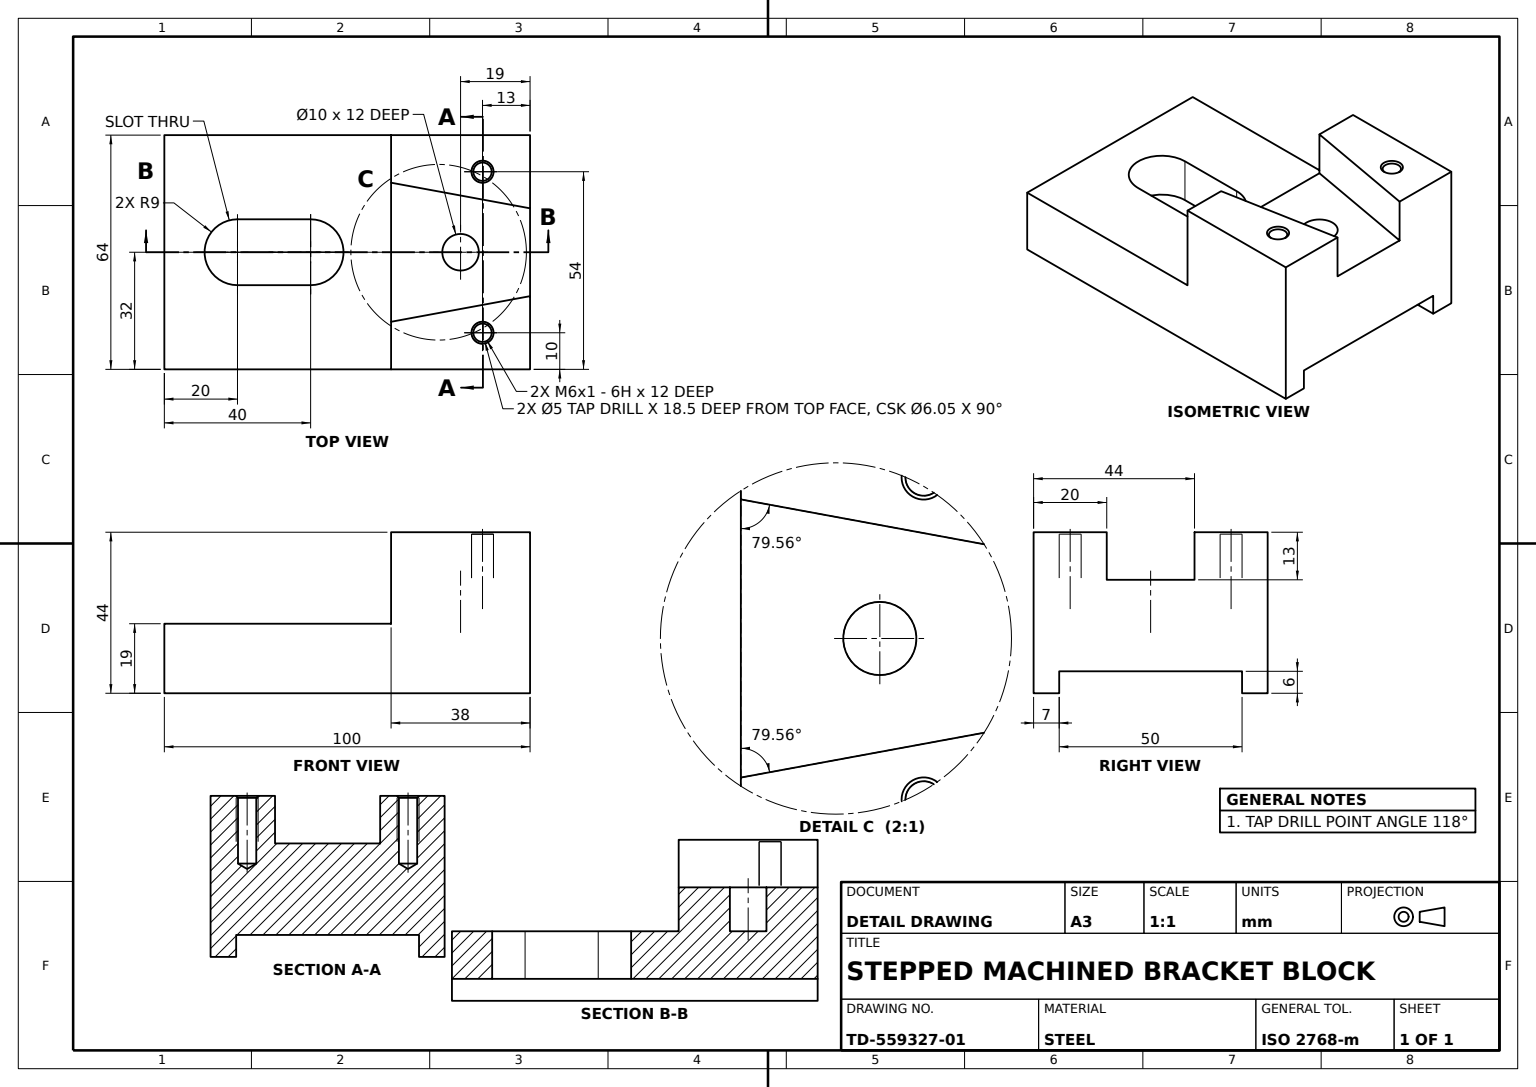
SolidWorks part; units mm, degrees
material "Plain Carbon Steel"
ref_plane "Front Plane" through (0, 0, 0) normal (0, 0, 1) x (1, 0, 0)
ref_plane "Top Plane" through (0, 0, 0) normal (0, 1, 0) x (1, 0, 0)
ref_plane "Right Plane" through (0, 0, 0) normal (1, 0, 0) x (0, 0, -1)
sketch "Base Plate Profile" plane through (0, 0, 0) normal (0, 0, 1) x (1, 0, 0)
  line L0 (25, 0) -> (-25, 0)
  line L1 (-25, 0) -> (-25, -6)
  line L2 (-25, -6) -> (-32, -6)
  line L3 (-32, -6) -> (-32, 13)
  line L4 (-32, 13) -> (32, 13)
  line L5 (32, 13) -> (32, -6)
  line L6 (32, -6) -> (25, -6)
  line L7 (25, -6) -> (25, 0)
  point P4 (0, 0)
  dimension "D1" = 50
  dimension "D2" = 19
  dimension "D3" = 7
  dimension "D4" = 6
  dimension "D5" = 6
  dimension "D6" = 7
  dimension "D7" = 64
extrude "Base Plate" add sketch "Base Plate Profile" against normal blind 100
sketch "V-Block Uprights Profile" plane through (0, 13, 0) normal (0, 1, 0) x (1, 0, 0)
  line L0 (32, 100) -> (32, 62)
  line L1 (32, 100) -> (32, 0) construction
  line L2 (32, 62) -> (19, 62)
  line L3 (19, 62) -> (12, 100)
  line L4 (32, 100) -> (-32, 100) construction
  line L5 (12, 100) -> (32, 100)
  line L6 (0, -24.2) -> (0, 24.2) construction
  line L7 (-12, 100) -> (-32, 100)
  line L8 (-32, 100) -> (-32, 62)
  line L9 (-32, 62) -> (-19, 62)
  line L10 (-19, 62) -> (-12, 100)
  dimension "D1" = 13
  dimension "D2" = 38
  dimension "D3" = 20
extrude "V-Block Uprights" add sketch "V-Block Uprights Profile" along normal blind 25
hole_wizard "M6 Tapped Holes 2x" positions "Sketch4" profile "Sketch5" tap size "M6" standard "ISO"
sketch "Sketch4" plane through (0, 38, 0) normal (0, 1, 0) x (1, 0, 0)
  line L0 (32, 62) -> (32, 100) construction
  line L1 (32, 100) -> (12, 100) construction
  line L2 (-32, 100) -> (-32, 62) construction
  line L3 (-12, 100) -> (-32, 100) construction
  point P0 (22, 87)
  point P2 (-22, 87)
  dimension "D1" = 10
  dimension "D2" = 13
  dimension "D3" = 10
  dimension "D4" = 13
sketch "Sketch5" plane through (22, 38, -87) normal (1, 0, 0) x (0, 0, 1)
  line L0 (0, 0) -> (0, 20)
  line L1 (0, 20) -> (2.5, 18.4978)
  line L2 (2.5, 18.4978) -> (2.5, 0.525)
  line L3 (2.5, 0.525) -> (3.025, 0)
  line L5 (3.025, 0) -> (0, 0)
  line L6 (-2.5, 0.525) -> (-3.025, 0) construction
  line L10 (0, 20) -> (-2.5, 18.4978) construction
  line L11 (0, -6.35) -> (0, 107.95) construction
  dimension "Tap Drill Dia." = 5
  dimension "Tap Drill Depth" = 20
  dimension "Near C'Sink Dia." = 6.05
  dimension "Near C'Sink Angle" = 90
  dimension "Drill Angle" = 118
cosmetic thread "Hole Thread1" parameters "D1"=12, "D2"=6
cosmetic thread "Hole Thread2" parameters "D1"=12, "D2"=6
sketch "Centre Step Block Profile" plane through (0, 13, 0) normal (0, 1, 0) x (1, 0, 0)
  line L0 (-12, 100) -> (12, 100)
  line L1 (12, 100) -> (19, 62)
  line L2 (19, 62) -> (-19, 62)
  line L3 (-19, 62) -> (-12, 100)
  circle A0 centre (0, 81) radius 5
  dimension "D1" = 19
  dimension "D3" = 10
  dimension "D2" = 12
extrude "Centre Step Block" add sketch "Centre Step Block Profile" along normal blind 12
sketch "Adjustment Slot and Centre Hole Profile" plane through (0, 13, 0) normal (0, 1, 0) x (1, 0, 0)
  line L0 (0, 20) -> (0, 40) construction
  line L1 (-9, 20) -> (-9, 40)
  line L2 (9, 20) -> (9, 40)
  line L3 (-19, 62) -> (19, 62) construction
  arc A0 (-9, 20) -> (9, 20) centre (0, 20) ccw
  arc A1 (9, 40) -> (-9, 40) centre (0, 40) ccw
  point P2 (0, 30)
  point P8 (-9, 30)
  point P11 (0, 49)
  dimension "D1" = 9
  dimension "D2" = 18
  dimension "D3" = 20
  dimension "D4" = 13
extrude "Adjustment Slot and Centre Hole" cut sketch "Adjustment Slot and Centre Hole Profile" against normal through all
